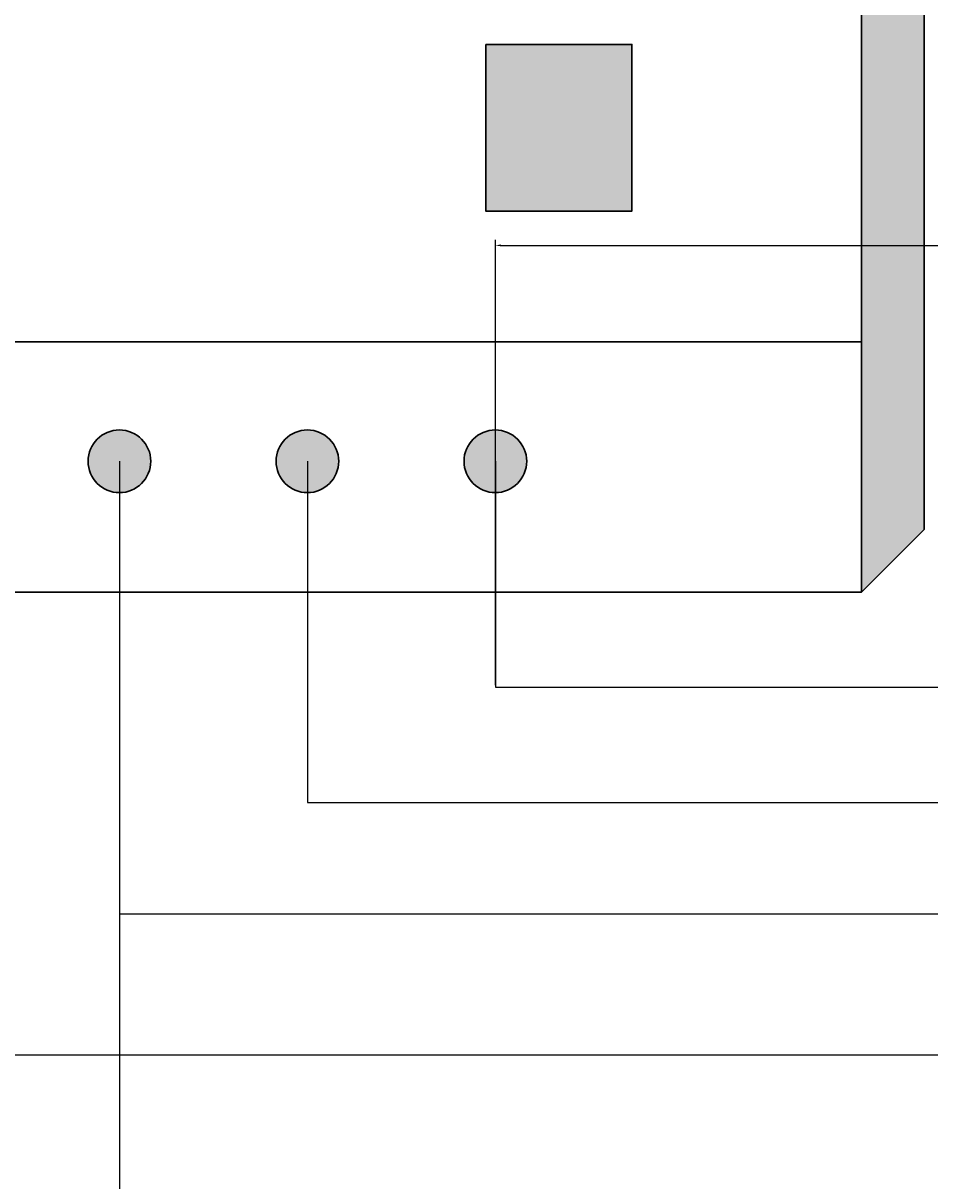
# Model space of a CAD drawing. Units: millimetres. Extents: x -8 to 285, y 5 to 221.
# Tile 6 of 30: x 55 to 84, y 45 to 82. Entities that reach past the tile are written whole.
import ezdxf

# ---------------------------------------------------------------- set-up
doc = ezdxf.new("R2010")
doc.units = ezdxf.units.MM
for name, color, linetype, lineweight in [('A-ANNO-DIMS', 2, 'Continuous', 18), ('E-EQPM-PATT', 252, 'Continuous', 13), ('E-POWR-CTRL', 7, 'Continuous', 30), ('E-POWR-DC-NEG', 3, 'Continuous', 25)]:
    doc.layers.add(name, color=color, linetype=linetype, lineweight=lineweight)
doc.layers.add('E-POWR-DC-POS', color=30, linetype='Continuous', lineweight=25, true_color=0xf26722)
doc.styles.get("Standard").update_dxf_attribs({"font": 'arial.ttf'})
doc.dimstyles.get("Standard").update_dxf_attribs({"dimtxt": 0.18, "dimasz": 0.18, "dimexe": 0.18, "dimexo": 0.0625, "dimgap": 0.09, "dimtad": 0, "dimtih": 1, "dimtoh": 1, "dimdec": 4, "dimzin": 0, "dimdsep": 46, "dimtxsty": 'Standard', "dimcen": 0.09, "dimadec": 0, "dimazin": 0, "dimtfac": 1, "dimtdec": 4, "dimtofl": 0, "dimtmove": 0, "dimatfit": 3, "dimfxl": 1, "dimtolj": 1, "dimtzin": 0, "dimarcsym": 0})

# ---------------------------------------------------------------- blocks, each defined once
blk = doc.blocks.new('*D10')
at = {"layer": 'A-ANNO-DIMS', "color": 0, "lineweight": -2, "transparency": 16777216}
for p, q in [((145.103, 206.457), (-7.608, 206.457)), ((-7.428, 206.277), (-7.428, 113.161)), ((-7.428, 19.682), (-7.428, 112.797)), ((30.453, 19.502), (-7.608, 19.502))]:
    blk.add_line(p, q, dxfattribs=at)
at = {"layer": 'A-ANNO-DIMS', "color": 0, "transparency": 16777216}
for points in [[(-7.458, 206.277), (-7.398, 206.277), (-7.428, 206.457)], [(-7.458, 19.682), (-7.398, 19.682), (-7.428, 19.502)]]:
    blk.add_solid(points, dxfattribs=at)
at = {"layer": 'Defpoints', "color": 0, "transparency": 16777216}
for p in [(-7.428, 206.457), (145.165, 206.457), (30.516, 19.502)]:
    blk.add_point(p, dxfattribs=at)
at = {"layer": 'A-ANNO-DIMS', "color": 0, "transparency": 16777216, "insert": (-7.428, 112.979), "char_height": 0.18, "attachment_point": 5}
blk.add_mtext('\\A1;186.95', dxfattribs=at)
blk = doc.blocks.new('*D25')
at = {"layer": 'A-ANNO-DIMS', "color": 0, "lineweight": -2, "transparency": 16777216}
for p, q in [((70.172, 60.759), (70.172, 74.977)), ((70.352, 74.797), (92.199, 74.797)), ((114.842, 74.797), (92.995, 74.797)), ((115.022, 60.759), (115.022, 74.977))]:
    blk.add_line(p, q, dxfattribs=at)
at = {"layer": 'A-ANNO-DIMS', "color": 0, "transparency": 16777216}
for points in [[(70.352, 74.827), (70.352, 74.767), (70.172, 74.797)], [(114.842, 74.827), (114.842, 74.767), (115.022, 74.797)]]:
    blk.add_solid(points, dxfattribs=at)
at = {"layer": 'Defpoints', "color": 0, "transparency": 16777216}
for p in [(115.022, 74.797), (70.172, 60.697), (115.022, 60.697)]:
    blk.add_point(p, dxfattribs=at)
at = {"layer": 'A-ANNO-DIMS', "color": 0, "transparency": 16777216, "insert": (92.597, 74.797), "char_height": 0.18, "attachment_point": 5}
blk.add_mtext('\\A1;44.85', dxfattribs=at)

msp = doc.modelspace()

# ---------------------------------------------------------------- hatches: boundary and pattern name
at = {"layer": 'E-EQPM-PATT'}
h = msp.add_hatch(color=256, dxfattribs=at)
h.set_gradient(color2=(0, 0, 0), tint=1)
h.paths.add_polyline_path([(41.1717, 67.9064, 1), (39.1717, 67.9064, 1)])
h.paths.add_polyline_path([(47.1717, 67.9064, 1), (45.1717, 67.9064, 1)])
h.paths.add_polyline_path([(53.1717, 67.9064, 1), (51.1717, 67.9064, 1)])
h.paths.add_polyline_path([(57.1717, 67.9064, 1), (59.1717, 67.9064, 1)])
h.paths.add_polyline_path([(65.1717, 67.9064, 1), (63.1717, 67.9064, 1)])
h.paths.add_polyline_path([(69.1717, 67.9064, 1), (71.1717, 67.9064, 1)])
h.paths.add_polyline_path([(148.1394, 196.6424), (148.1394, 201.7939), (142.1909, 201.7939), (142.1909, 196.6424)])
h.paths.add_polyline_path([(186.1388, 201.7939), (186.1388, 196.6424), (192.0873, 196.6424), (192.0873, 201.7939)])
h.paths.add_polyline_path([(234.0155, 196.6424), (234.0155, 201.7939), (228.067, 201.7939), (228.067, 196.6424)])
h = msp.add_hatch(color=256, dxfattribs=at)
h.set_gradient(color1=(248, 153, 30), color2=(248, 153, 30), tint=1)
h.paths.add_polyline_path([(28.1554, 99.1437), (26.1554, 97.1437), (26.1554, 65.7282), (28.0483, 63.8353)])
h.paths.add_polyline_path([(81.859, 63.7282), (83.859, 65.7282), (83.859, 97.1437), (81.859, 99.1437)])
h.paths.add_polyline_path([(39.086, 92.2191), (34.4177, 92.2191), (34.4177, 86.904), (39.086, 86.904)])
h.paths.add_polyline_path([(74.424, 86.904), (74.424, 92.2191), (69.7557, 92.2191), (69.7557, 86.904)])
h.paths.add_polyline_path([(74.5326, 81.2093), (69.8643, 81.2093), (69.8643, 75.8943), (74.5326, 75.8943)])
h.paths.add_polyline_path([(34.4177, 75.3519), (39.086, 75.3519), (39.086, 80.667), (34.4177, 80.667)])

# ---------------------------------------------------------------- linework, layer by layer
at = {"layer": 'E-POWR-CTRL'}
for p, q in [((81.859, 99.1437), (81.859, 63.7282)), ((28.0722, 71.7183), (81.859, 71.7183))]:
    msp.add_line(p, q, dxfattribs=at)
for points in [[(28.1554, 99.1437), (81.859, 99.1437), (83.859, 97.1437), (83.859, 65.7282), (81.859, 63.7282), (28.1554, 63.7282), (26.1554, 65.7282), (26.1554, 97.1437)], [(69.8643, 81.2093), (74.5326, 81.2093), (74.5326, 75.8943), (69.8643, 75.8943)]]:
    msp.add_lwpolyline(points, close=True, dxfattribs=at)
for centre in [(58.1717, 67.9064), (64.1717, 67.9064), (70.1717, 67.9064)]:
    msp.add_circle(centre, 1, dxfattribs=at)
at = {"layer": 'E-POWR-DC-NEG'}
msp.add_line((58.1717, 53.4644), (215.8749, 53.4644), dxfattribs=at)
for points in [[(70.1717, 67.9064), (70.1717, 60.6968), (115.0224, 60.6968), (115.0224, 91.5754)], [(58.1717, 67.9064), (58.1717, 43.2239), (94.0348, 43.2239), (94.1079, 38.4537)]]:
    msp.add_lwpolyline(points, dxfattribs=at)
at = {"layer": 'E-POWR-DC-POS'}
for points in [[(64.1717, 67.9064), (64.1717, 57.0172), (124.134, 57.0172), (124.134, 93.361)], [(52.1717, 48.962), (202.4345, 48.962), (202.4345, 34.9746)]]:
    msp.add_lwpolyline(points, dxfattribs=at)

# ---------------------------------------------------------------- dimensions: what is measured, and where the dimension line sits
at = {"layer": 'A-ANNO-DIMS'}
dim = msp.add_linear_dim(base=(-7.4275, 206.4568), p1=(30.516, 19.502), p2=(145.1651, 206.4568), angle=90, dimstyle='Standard', override={"dimdec": 2, "dimlfac": 1, "dimrnd": 0, "dimzin": 0, "dimdsep": 46, "dimlunit": 2}, dxfattribs=at)
dim.commit()
dim.dimension.update_dxf_attribs({"geometry": '*D10', "text_midpoint": (-7.4275, 112.9794)})
dim = msp.add_linear_dim(base=(115.0224, 74.7968), p1=(70.1717, 60.6968), p2=(115.0224, 60.6968), dimstyle='Standard', override={"dimdec": 2, "dimlfac": 1, "dimrnd": 0, "dimzin": 0, "dimdsep": 46, "dimlunit": 2}, dxfattribs=at)
dim.commit()
dim.dimension.update_dxf_attribs({"geometry": '*D25', "text_midpoint": (92.597, 74.7968)})

doc.saveas('drawing.dxf')
